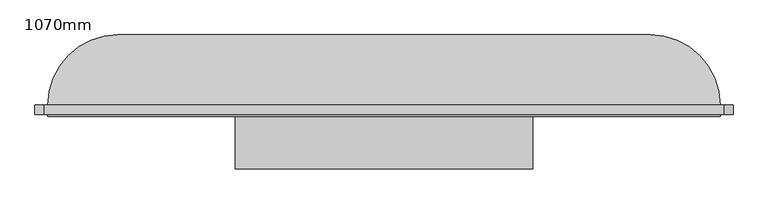
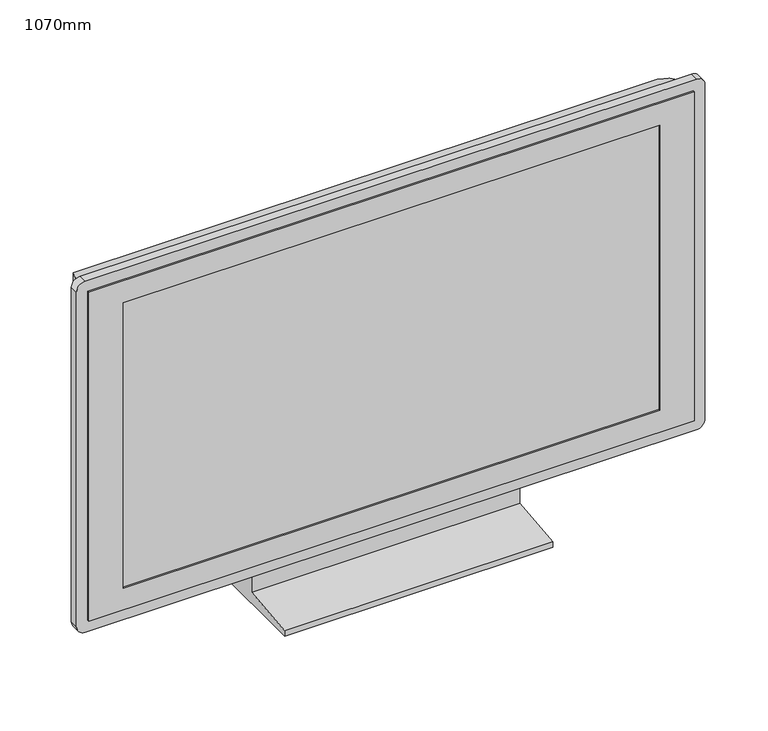
"""IFC4 building model written with IfcOpenShell, lengths in millimetres: furniture geometry, 1070mm."""

from ifc_helpers import new_model, si_unit, point, frame, frame_2d, origin, place, context, project, spatial, polyline, circle_curve, ellipse_curve, trimmed, segment, composite_curve, outline, extrude, faceted_brep, source, transform, mapped, element, save
from ifc_brep_helpers import plane_surface, cylinder_surface, advanced_brep


def furniture_1070mm_7a3aaa4f(model_context):
    return source(origin(), model_context, "Body", "SolidModel", [
        extrude(outline(polyline([(-51.4613764, 80.0), (-1.4613764, 80.0), (48.5386236, 0.0), (-151.4613764, 0.0), (-151.4613764, 10.0), (-51.4613764, 20.0), (-51.4613764, 80.0)])), frame((-237.0858282, 0.0, 0.0), z_axis=(1.0, 0.0, 0.0), x_axis=(0.0, 1.0, 0.0)), (0.0, 0.0, 1.0), 466.2826281),
        faceted_brep([(522.338114, -69.4613764, 684.6160909), (-530.2271423, -69.4613764, 684.6160909), (-530.2271423, -69.4613764, 80.0), (522.338114, -69.4613764, 80.0), (-470.2271423, -69.4613764, 644.6160909), (462.338114, -69.4613764, 644.6160909), (462.338114, -69.4613764, 120.0), (-470.2271423, -69.4613764, 120.0), (522.338114, -51.4613764, 684.6160909), (522.338114, -51.4613764, 80.0), (-530.2271423, -51.4613764, 80.0), (-530.2271423, -51.4613764, 684.6160909), (-470.2271423, -66.4613764, 644.6160909), (-470.2271423, -66.4613764, 120.0), (462.338114, -66.4613764, 120.0), (462.338114, -66.4613764, 644.6160909)], [[[0, 1, 2, 3], [4, 5, 6, 7]], [[8, 9, 10, 11]], [[1, 0, 8, 11]], [[2, 1, 11, 10]], [[3, 2, 10, 9]], [[0, 3, 9, 8]], [[12, 13, 14, 15]], [[12, 15, 5, 4]], [[15, 14, 6, 5]], [[14, 13, 7, 6]], [[13, 12, 4, 7]]]),
        extrude(outline(composite_curve([segment(polyline([(704.6160909, 527.338114), (704.6160909, -535.2271423)]), True, "CONTINUOUS"), segment(trimmed(circle_curve(frame_2d((689.6160909, -535.2271423)), 15.0), [point((704.6160909, -535.2271423))], [point((689.6160909, -550.2271423))], False, "CARTESIAN"), True, "CONTINUOUS"), segment(polyline([(689.6160909, -550.2271423), (75.0, -550.2271423)]), True, "CONTINUOUS"), segment(trimmed(circle_curve(frame_2d((75.0, -535.2271423)), 15.0), [point((75.0, -550.2271423))], [point((60.0, -535.2271423))], False, "CARTESIAN"), True, "CONTINUOUS"), segment(polyline([(60.0, -535.2271423), (60.0, 527.338114)]), True, "CONTINUOUS"), segment(trimmed(circle_curve(frame_2d((75.0, 527.338114)), 15.0), [point((60.0, 527.338114))], [point((75.0, 542.338114))], False, "CARTESIAN"), True, "CONTINUOUS"), segment(polyline([(75.0, 542.338114), (689.6160909, 542.338114)]), True, "CONTINUOUS"), segment(trimmed(circle_curve(frame_2d((689.6160909, 527.338114)), 15.0), [point((689.6160909, 542.338114))], [point((704.6160909, 527.338114))], False, "CARTESIAN"), True, "CONTINUOUS")], self_intersect=False), holes=[polyline([(684.6160909, 522.338114), (80.0, 522.338114), (80.0, -530.2271423), (684.6160909, -530.2271423), (684.6160909, 522.338114)])]), frame((0.0, -66.4613764, 0.0), z_axis=(0.0, 1.0, 0.0), x_axis=(0.0, 0.0, 1.0)), (0.0, 0.0, 1.0), 15.0),
        advanced_brep(
        [(-530.2271423, -51.4613764, 80.0), (522.338114, -51.4613764, 80.0), (522.338114, -51.4613764, 684.6160909), (-530.2271423, -51.4613764, 684.6160909), (412.338114, 58.5386236, 80.0), (-420.2271423, 58.5386236, 80.0), (-420.2271423, 58.5386236, 574.6160909), (412.338114, 58.5386236, 574.6160909)],
        [
            (0, 1),
            (1, 2),
            (2, 3),
            (3, 0),
            (4, 5),
            (5, 6),
            (6, 7),
            (7, 4),
            (0, 5, circle_curve(frame((-420.2271423, -51.4613764, 80.0), z_axis=(0.0, 0.0, -1.0), x_axis=(-1.0, 0.0, 0.0)), 110.0)),
            (4, 1, circle_curve(frame((412.338114, -51.4613764, 80.0), z_axis=(0.0, 0.0, -1.0), x_axis=(1.0, 0.0, 0.0)), 110.0)),
            (7, 2, ellipse_curve(frame((412.338114, -51.4613764, 574.6160909), z_axis=(0.7071067811865475, 0.0, -0.7071067811865475), x_axis=(0.7071067811865474, 0.0, 0.7071067811865476)), 155.5634919, 110.0)),
            (6, 3, ellipse_curve(frame((-420.2271423, -51.4613764, 574.6160909), z_axis=(0.7071067811865475, 0.0, 0.7071067811865475), x_axis=(-0.7071067811865476, 0.0, 0.7071067811865474)), 155.5634919, 110.0)),
        ],
        [
            plane_surface(frame((-530.2271423, -51.4613764, 684.6160909), z_axis=(0.0, -1.0, 0.0), x_axis=(-1.0, 0.0, 0.0))),
            plane_surface(frame((-530.2271423, 58.5386236, 684.6160909), z_axis=(0.0, 1.0, 0.0), x_axis=(1.0, 0.0, 0.0))),
            plane_surface(frame((-530.2271423, -51.4613764, 80.0), z_axis=(0.0, 0.0, -1.0), x_axis=(0.0, 1.0, 0.0))),
            cylinder_surface(frame((412.338114, -51.4613764, 80.0), z_axis=(0.0, 0.0, 1.0), x_axis=(1.0, 0.0, 0.0)), 110.0),
            cylinder_surface(frame((522.338114, -51.4613764, 574.6160909), z_axis=(-1.0, 0.0, 0.0), x_axis=(0.0, 0.0, 1.0)), 110.0),
            cylinder_surface(frame((-420.2271423, -51.4613764, 684.6160909), z_axis=(0.0, 0.0, -1.0), x_axis=(-1.0, 0.0, 0.0)), 110.0),
        ],
        [
            (0, [[1, 2, 3, 4]]),
            (1, [[5, 6, 7, 8]]),
            (2, [[-1, 9, -5, 10]]),
            (3, [[11, -2, -10, -8]]),
            (4, [[-11, -7, 12, -3]]),
            (5, [[-12, -6, -9, -4]]),
        ],
    ),
    ])


if __name__ == "__main__":
    model = new_model("IFC4")
    model_context = context("Model", 3, world=origin())
    ifc_project = project(units=[si_unit("LENGTHUNIT", "METRE", prefix="MILLI")], contexts=[model_context])
    site = spatial("IfcSite", under=ifc_project)
    building = spatial("IfcBuilding", under=site)
    placement = place(None, origin())
    furniture_1070mm_shape = furniture_1070mm_7a3aaa4f(model_context)
    element("IfcFurniture", 1, ObjectType="1070mm", at=placement, inside=building, context=model_context, shape_type="MappedRepresentation", body=[
        mapped(furniture_1070mm_shape, transform((0.0, 0.0, 0.0), x_axis=(1.0, 0.0, 0.0), y_axis=(0.0, 1.0, 0.0), z_axis=(0.0, 0.0, 1.0))),
    ])
    save(model, "model.ifc")

# Revit data of these elements
# Type "1070mm"
#   SinAng = 0' - 0.0193"
#   L = 3' - 0.71517"
#   H = 1' - 8.65418"
#   Thickness = 0' - 4.33071"
#   Diagonal = 3' - 6.12598"
#   CosAng = 0' - 0.03431"
#   Stand [instance default] = yes
#   Default Elevation = 0
# Element 1 (IfcFurniture, "1070mm")
#   Materials on its faces: "TV - Black", "TV - Glass", "TV - Screen"
# Materials
#   "TV - Black": colour RGB 49 49 49, transparency 0
#   "TV - Glass": colour RGB 157 157 157, transparency 0.9
#   "TV - Screen": colour RGB 0 0 0, transparency 0
